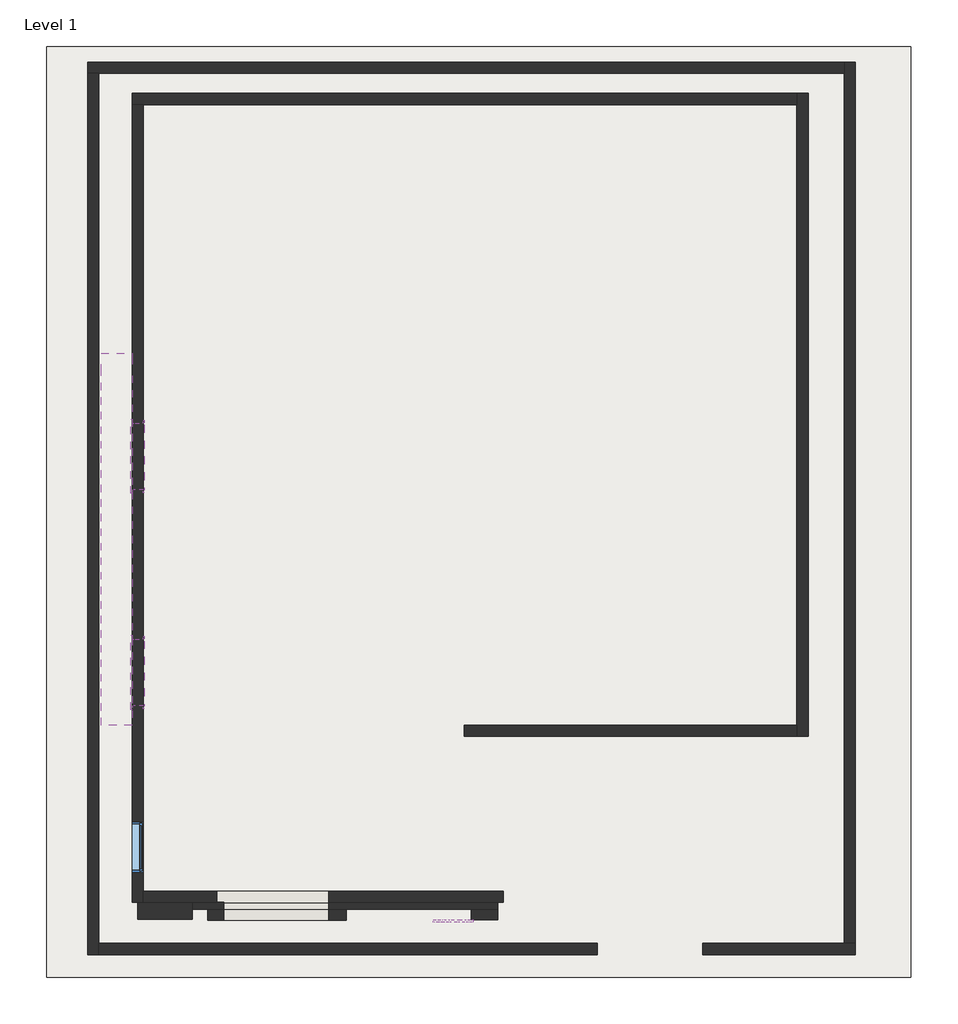
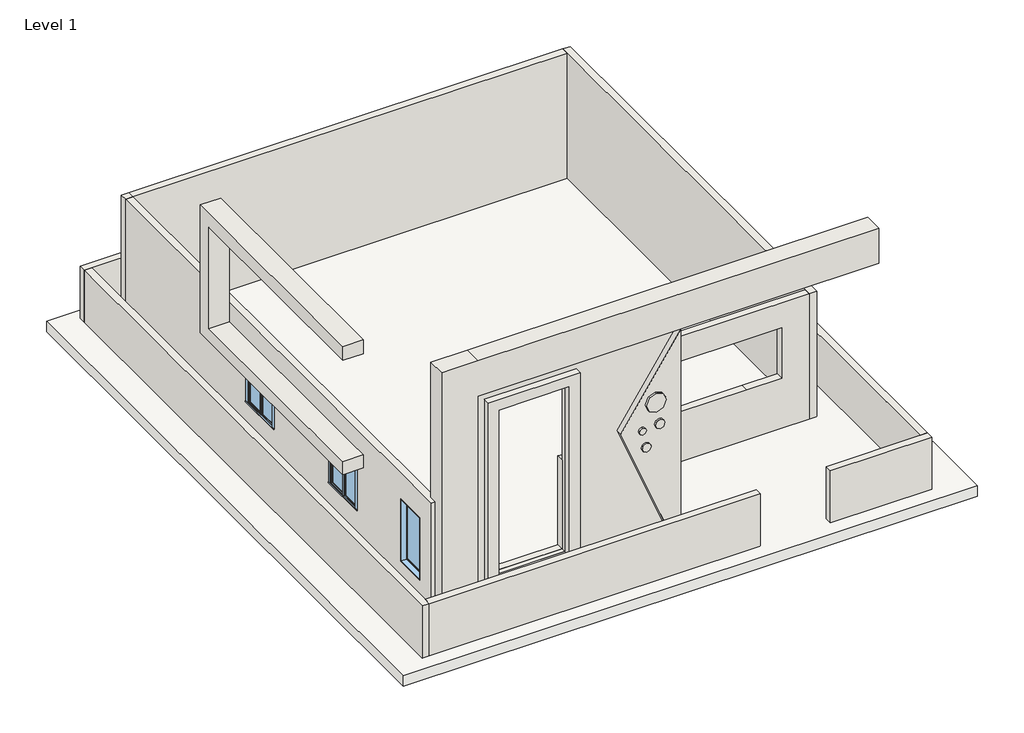
# One storey: 15 walls, 3 windows, 1 slab.
"""IFC4 building model written with IfcOpenShell, lengths in millimetres."""

from ifc_helpers import new_model, si_unit, frame, origin, place, context, project, spatial, polyline, outline, extrude, faceted_brep, transform, mapped, element, save
from components import walls_1_walls_1_592a891f, walls_3_walls_3_f969b8b6, walls_4_walls_4_f4f7f16f, walls_5_walls_5_14261912, walls_6_walls_6_dde418cc, walls_7_walls_7_556ff675, window_0862ab64, window_9a779fa2

model = new_model("IFC4")

# Units and contexts
model_context = context("Model", 3, world=origin())
ifc_project = project(units=[si_unit("LENGTHUNIT", "METRE", prefix="MILLI")], contexts=[model_context])

# Site, building, storey
site = spatial("IfcSite", under=ifc_project)
building = spatial("IfcBuilding", under=site)
storey = spatial("IfcBuildingStorey", under=building, Name="Level 1", Elevation=0.0)

# Slab
placement = place(None, origin())
element("IfcSlab", 1, ObjectType="Generic - 12\"", at=placement, inside=storey, context=model_context, shape_type="SweptSolid", body=[
    extrude(outline(polyline([(5705.2565279, 11449.004673), (5705.2565279, -5619.795327), (-10144.3434721, -5619.795327), (-10144.3434721, 11449.004673), (5705.2565279, 11449.004673)])), frame((0.0, 0.0, -304.8), z_axis=(0.0, 0.0, 1.0), x_axis=(1.0, 0.0, 0.0)), (0.0, 0.0, 1.0), 304.8),
])

# Walls
element("IfcWall", 2, ObjectType="Generic - 8\"", at=placement, inside=storey, context=model_context, shape_type="Brep", body=[
    faceted_brep([(-8577.2311901, 10384.6860488, 0.0), (-8374.0311901, 10384.6860488, 0.0), (3614.7688099, 10384.6860488, 0.0), (3614.7688099, 10384.6860488, 3657.6), (-8374.0311901, 10384.6860488, 3657.6), (-8577.2311901, 10384.6860488, 3657.6), (-8577.2311901, 10587.8860488, 0.0), (-8577.2311901, 10587.8860488, 3657.6), (-8374.0311901, 10587.8860488, 3657.6), (3614.7688099, 10587.8860488, 3657.6), (3614.7688099, 10587.8860488, 0.0)], [[[0, 1, 2, 3, 4, 5]], [[6, 7, 8, 9, 10]], [[2, 1, 0, 6, 10]], [[0, 5, 7, 6]], [[3, 2, 10, 9]], [[5, 4, 8, 7]], [[4, 3, 9, 8]]]),
])
element("IfcWall", 3, ObjectType="Generic - 8\"", at=placement, inside=storey, context=model_context, shape_type="Brep", body=[
    faceted_brep([(-8374.0311901, -4245.7139512, 0.0), (-8374.0311901, -4042.5139512, 0.0), (-8374.0311901, 10384.6860488, 0.0), (-8374.0311901, 10384.6860488, 3657.6), (-8374.0311901, -4042.5139512, 3657.6), (-8374.0311901, -4245.7139512, 3657.6), (-8374.0311901, -3686.9139512, 2900.7966345), (-8374.0311901, -2772.5139512, 2900.7966345), (-8374.0311901, -2772.5139512, 1071.9966345), (-8374.0311901, -3686.9139512, 1071.9966345), (-8374.0311901, 4542.6860488, 2485.5847354), (-8374.0311901, 4542.6860488, 1266.3847354), (-8374.0311901, 3323.4860488, 1266.3847354), (-8374.0311901, 3323.4860488, 2485.5847354), (-8374.0311901, 580.2860488, 2522.8889162), (-8374.0311901, 580.2860488, 1303.6889162), (-8374.0311901, -638.9139512, 1303.6889162), (-8374.0311901, -638.9139512, 2522.8889162), (-8577.2311901, -4245.7139512, 0.0), (-8577.2311901, -4245.7139512, 3657.6), (-8577.2311901, 10384.6860488, 3657.6), (-8577.2311901, 10384.6860488, 0.0), (-8577.2311901, -3686.9139512, 2900.7966345), (-8577.2311901, -3686.9139512, 1071.9966345), (-8577.2311901, -2772.5139512, 1071.9966345), (-8577.2311901, -2772.5139512, 2900.7966345), (-8577.2311901, 4542.6860488, 2485.5847354), (-8577.2311901, 3323.4860488, 2485.5847354), (-8577.2311901, 3323.4860488, 1266.3847354), (-8577.2311901, 4542.6860488, 1266.3847354), (-8577.2311901, 580.2860488, 2522.8889162), (-8577.2311901, -638.9139512, 2522.8889162), (-8577.2311901, -638.9139512, 1303.6889162), (-8577.2311901, 580.2860488, 1303.6889162)], [[[0, 1, 2, 3, 4, 5], [6, 7, 8, 9], [10, 11, 12, 13], [14, 15, 16, 17]], [[18, 19, 20, 21], [22, 23, 24, 25], [26, 27, 28, 29], [30, 31, 32, 33]], [[2, 1, 0, 18, 21]], [[5, 4, 3, 20, 19]], [[0, 5, 19, 18]], [[3, 2, 21, 20]], [[23, 22, 6, 9]], [[24, 23, 9, 8]], [[25, 24, 8, 7]], [[22, 25, 7, 6]], [[11, 10, 26, 29]], [[12, 11, 29, 28]], [[13, 12, 28, 27]], [[10, 13, 27, 26]], [[15, 14, 30, 33]], [[16, 15, 33, 32]], [[17, 16, 32, 31]], [[14, 17, 31, 30]]]),
])
element("IfcWall", 4, ObjectType="Generic - 8\"", at=placement, inside=storey, context=model_context, shape_type="Brep", body=[
    faceted_brep([(-1770.0311901, -4042.5139512, 0.0), (-8374.0311901, -4042.5139512, 0.0), (-8374.0311901, -4042.5139512, 3657.6), (-7057.7216902, -4042.5139512, 3657.6), (-7024.8824762, -4042.5139512, 3657.6), (-7024.8824762, -4042.5139512, 1066.8), (-4972.3150386, -4042.5139512, 1066.8), (-4972.3150386, -4042.5139512, 3657.6), (-4944.6813589, -4042.5139512, 3657.6), (-1871.6311901, -4042.5139512, 3657.6), (-1770.0311901, -4042.5139512, 3657.6), (-1770.0311901, -4245.7139512, 0.0), (-1770.0311901, -4245.7139512, 3657.6), (-1871.6311901, -4245.7139512, 3657.6), (-4944.6813589, -4245.7139512, 3657.6), (-4972.3150386, -4245.7139512, 3657.6), (-4972.3150386, -4245.7139512, 1066.8), (-7024.8824762, -4245.7139512, 1066.8), (-7024.8824762, -4245.7139512, 3657.6), (-7057.7216902, -4245.7139512, 3657.6), (-8374.0311901, -4245.7139512, 3657.6), (-8374.0311901, -4245.7139512, 0.0)], [[[0, 1, 2, 3, 4, 5, 6, 7, 8, 9, 10]], [[11, 12, 13, 14, 15, 16, 17, 18, 19, 20, 21]], [[2, 1, 21, 20]], [[1, 0, 11, 21]], [[0, 10, 12, 11]], [[4, 3, 2, 20, 19, 18]], [[5, 4, 18, 17]], [[6, 5, 17, 16]], [[7, 6, 16, 15]], [[9, 8, 7, 15, 14, 13]], [[10, 9, 13, 12]]]),
])
element("IfcWall", 5, ObjectType="Generic - 8\"", at=placement, inside=storey, context=model_context, shape_type="Brep", body=[
    faceted_brep([(3614.7688099, 10587.8860488, 0.0), (3614.7688099, 10384.6860488, 0.0), (3614.7688099, -994.5139512, 0.0), (3614.7688099, -1197.7139512, 0.0), (3614.7688099, -1197.7139512, 3657.6), (3614.7688099, -994.5139512, 3657.6), (3614.7688099, 10384.6860488, 3657.6), (3614.7688099, 10587.8860488, 3657.6), (3817.9688099, 10587.8860488, 0.0), (3817.9688099, 10587.8860488, 3657.6), (3817.9688099, -1197.7139512, 3657.6), (3817.9688099, -1197.7139512, 0.0)], [[[0, 1, 2, 3, 4, 5, 6, 7]], [[8, 9, 10, 11]], [[3, 2, 1, 0, 8, 11]], [[0, 7, 9, 8]], [[7, 6, 5, 4, 10, 9]], [[4, 3, 11, 10]]]),
])
element("IfcWall", 6, ObjectType="Generic - 8\"", at=placement, inside=storey, context=model_context, shape_type="SweptSolid", body=[
    extrude(outline(polyline([(0.0, 3614.7688099), (3657.6, 3614.7688099), (3657.6, -2481.2311901), (0.0, -2481.2311901), (0.0, 3614.7688099)]), holes=[polyline([(2930.097392, 2852.2278443), (1465.048696, 2852.2278443), (1465.048696, 1887.5688099), (1465.048696, -1052.1762723), (2930.097392, -1052.1762723), (2930.097392, 2852.2278443)])]), frame((0.0, -1197.7139512, 0.0), z_axis=(0.0, 1.0, 0.0), x_axis=(0.0, 0.0, 1.0)), (0.0, 0.0, 1.0), 203.2),
])
element("IfcWall", 7, ObjectType="Generic - 8\"", at=placement, inside=storey, context=model_context, shape_type="Brep", body=[
    faceted_brep([(-9386.1684306, 10954.9442531, 0.0), (-9182.9684306, 10954.9442531, 0.0), (4482.2315694, 10954.9442531, 0.0), (4482.2315694, 10954.9442531, 1524.0), (-9182.9684306, 10954.9442531, 1524.0), (-9386.1684306, 10954.9442531, 1524.0), (-9386.1684306, 11158.1442531, 0.0), (-9386.1684306, 11158.1442531, 1524.0), (4482.2315694, 11158.1442531, 1524.0), (4482.2315694, 11158.1442531, 0.0)], [[[0, 1, 2, 3, 4, 5]], [[6, 7, 8, 9]], [[2, 1, 0, 6, 9]], [[5, 4, 3, 8, 7]], [[0, 5, 7, 6]], [[3, 2, 9, 8]]]),
])
element("IfcWall", 8, ObjectType="Generic - 8\"", at=placement, inside=storey, context=model_context, shape_type="Brep", body=[
    faceted_brep([(-9182.9684306, -5199.4557469, 0.0), (-9182.9684306, -4996.2557469, 0.0), (-9182.9684306, 10954.9442531, 0.0), (-9182.9684306, 10954.9442531, 1524.0), (-9182.9684306, -4996.2557469, 1524.0), (-9182.9684306, -5199.4557469, 1524.0), (-9386.1684306, -5199.4557469, 0.0), (-9386.1684306, -5199.4557469, 1524.0), (-9386.1684306, 10954.9442531, 1524.0), (-9386.1684306, 10954.9442531, 0.0)], [[[0, 1, 2, 3, 4, 5]], [[6, 7, 8, 9]], [[2, 1, 0, 6, 9]], [[5, 4, 3, 8, 7]], [[0, 5, 7, 6]], [[3, 2, 9, 8]]]),
])
element("IfcWall", 9, ObjectType="Generic - 8\"", at=placement, inside=storey, context=model_context, shape_type="Brep", body=[
    faceted_brep([(-9182.9684306, -4996.2557469, 1524.0), (-42.8311901, -4996.2557469, 1524.0), (-42.8311901, -4996.2557469, 0.0), (-9182.9684306, -4996.2557469, 0.0), (-9182.9684306, -5199.4557469, 1524.0), (-9182.9684306, -5199.4557469, 0.0), (-42.8311901, -5199.4557469, 0.0), (-42.8311901, -5199.4557469, 1524.0)], [[[0, 1, 2, 3]], [[4, 5, 6, 7]], [[0, 3, 5, 4]], [[1, 0, 4, 7]], [[2, 1, 7, 6]], [[3, 2, 6, 5]]]),
    faceted_brep([(4685.4315694, -4996.2557469, 0.0), (4482.2315694, -4996.2557469, 0.0), (1887.5688099, -4996.2557469, 0.0), (1887.5688099, -4996.2557469, 1524.0), (4482.2315694, -4996.2557469, 1524.0), (4685.4315694, -4996.2557469, 1524.0), (4685.4315694, -5199.4557469, 0.0), (4685.4315694, -5199.4557469, 1524.0), (1887.5688099, -5199.4557469, 1524.0), (1887.5688099, -5199.4557469, 0.0)], [[[0, 1, 2, 3, 4, 5]], [[6, 7, 8, 9]], [[0, 5, 7, 6]], [[2, 1, 0, 6, 9]], [[3, 2, 9, 8]], [[5, 4, 3, 8, 7]]]),
])
element("IfcWall", 10, ObjectType="Generic - 8\"", at=placement, inside=storey, context=model_context, shape_type="Brep", body=[
    faceted_brep([(4482.2315694, 11158.1442531, 0.0), (4482.2315694, 10954.9442531, 0.0), (4482.2315694, -4996.2557469, 0.0), (4482.2315694, -4996.2557469, 1524.0), (4482.2315694, 10954.9442531, 1524.0), (4482.2315694, 11158.1442531, 1524.0), (4685.4315694, 11158.1442531, 0.0), (4685.4315694, 11158.1442531, 1524.0), (4685.4315694, -4996.2557469, 1524.0), (4685.4315694, -4996.2557469, 0.0)], [[[0, 1, 2, 3, 4, 5]], [[6, 7, 8, 9]], [[2, 1, 0, 6, 9]], [[5, 4, 3, 8, 7]], [[0, 5, 7, 6]], [[3, 2, 9, 8]]]),
])
walls_1_walls_1_shape = walls_1_walls_1_592a891f(model_context)
element("IfcWall", 11, ObjectType="Walls 1 : Walls 1", at=placement, inside=storey, context=model_context, shape_type="MappedRepresentation", body=[
    mapped(walls_1_walls_1_shape, transform((0.0, 0.0, 0.0), x_axis=(1.0, 0.0, 0.0), y_axis=(0.0, 1.0, 0.0), z_axis=(0.0, 0.0, 1.0))),
])
walls_3_walls_3_shape = walls_3_walls_3_f969b8b6(model_context)
element("IfcWall", 12, ObjectType="Walls 3 : Walls 3", at=placement, inside=storey, context=model_context, shape_type="MappedRepresentation", body=[
    mapped(walls_3_walls_3_shape, transform((0.0, 0.0, 0.0), x_axis=(1.0, 0.0, 0.0), y_axis=(0.0, 1.0, 0.0), z_axis=(0.0, 0.0, 1.0))),
])
walls_4_walls_4_shape = walls_4_walls_4_f4f7f16f(model_context)
element("IfcWall", 13, ObjectType="Walls 4 : Walls 4", at=placement, inside=storey, context=model_context, shape_type="MappedRepresentation", body=[
    mapped(walls_4_walls_4_shape, transform((0.0, 0.0, 0.0), x_axis=(1.0, 0.0, 0.0), y_axis=(0.0, 1.0, 0.0), z_axis=(0.0, 0.0, 1.0))),
])
walls_5_walls_5_shape = walls_5_walls_5_14261912(model_context)
element("IfcWall", 14, ObjectType="Walls 5 : Walls 5", at=placement, inside=storey, context=model_context, shape_type="MappedRepresentation", body=[
    mapped(walls_5_walls_5_shape, transform((0.0, 0.0, 0.0), x_axis=(1.0, 0.0, 0.0), y_axis=(0.0, 1.0, 0.0), z_axis=(0.0, 0.0, 1.0))),
])
walls_6_walls_6_shape = walls_6_walls_6_dde418cc(model_context)
element("IfcWall", 15, ObjectType="Walls 6 : Walls 6", at=placement, inside=storey, context=model_context, shape_type="MappedRepresentation", body=[
    mapped(walls_6_walls_6_shape, transform((0.0, 0.0, 0.0), x_axis=(1.0, 0.0, 0.0), y_axis=(0.0, 1.0, 0.0), z_axis=(0.0, 0.0, 1.0))),
])
walls_7_walls_7_shape = walls_7_walls_7_556ff675(model_context)
element("IfcWall", 16, ObjectType="Walls 7 : Walls 7", at=placement, inside=storey, context=model_context, shape_type="MappedRepresentation", body=[
    mapped(walls_7_walls_7_shape, transform((0.0, 0.0, 0.0), x_axis=(1.0, 0.0, 0.0), y_axis=(0.0, 1.0, 0.0), z_axis=(0.0, 0.0, 1.0))),
])

# Windows
window_shape = window_0862ab64(model_context)
element("IfcWindow", 17, ObjectType="Casement Dbl with Trim : 48\" x 48\"", at=placement, inside=storey, context=model_context, shape_type="MappedRepresentation", body=[
    mapped(window_shape, transform((-8456.5811901, 3933.0860488, 351.9847354), x_axis=(0.0, 1.0, 0.0), y_axis=(-1.0, 0.0, 0.0), z_axis=(0.0, 0.0, 1.0))),
])
element("IfcWindow", 18, ObjectType="Casement Dbl with Trim : 48\" x 48\"", at=placement, inside=storey, context=model_context, shape_type="MappedRepresentation", body=[
    mapped(window_shape, transform((-8456.5811901, -29.3139512, 389.2889162), x_axis=(0.0, 1.0, 0.0), y_axis=(-1.0, 0.0, 0.0), z_axis=(0.0, 0.0, 1.0))),
])
window_2_shape = window_9a779fa2(model_context)
element("IfcWindow", 19, ObjectType="Fixed : 36\" x 72\"", at=placement, inside=storey, context=model_context, shape_type="MappedRepresentation", body=[
    mapped(window_2_shape, transform((-8475.6311901, -3267.8139512, 767.1966345), x_axis=(0.0, -1.0, 0.0), y_axis=(1.0, 0.0, 0.0), z_axis=(0.0, 0.0, 1.0))),
])

save(model, "model.ifc")

# Revit data of these elements
# Type "Generic - 12\""
#   Assembly Code = "B1010"
#   Function = 0
#   Layers, outside or top first: 1' - 0" no material (function 1)
# Type "Generic - 8\""
#   Assembly Code = "B2010"
#   Layers, outside or top first: 0' - 8" no material (function 1)
# Type "Casement Dbl with Trim : 48\" x 48\""
#   Type Mark = "10"
#   Construction Type Id = "GSP4R"
#   Assembly Code = "B2020100"
#   Analytic Construction = "1/8 in Pilkington single glazing"
#   Visual Light Transmittance = 0.9
#   Thermal Resistance (R) = 1.53941 (h·ft²·°F)/BTU
#   Solar Heat Gain Coefficient = 0.78
#   Heat Transfer Coefficient (U) = 0.6496 BTU/(h·ft²·°F)
#   Height = 4' - 0"
#   Default Sill Height = 3' - 0"
#   Trim Projection - Ext. = 0' - 0 1/2"
#   Trim Projection - Int. = 0' - 0 3/4"
#   Trim Width - Exterior = 0' - 3 1/2"
#   Trim Width - Interior = 0' - 3 1/2"
#   Width = 4' - 0"
#   Window Inset = 0' - 0 3/4"
#   Define Thermal Properties by = 1
#   Glass Pane Material = Glass
#   Sash Material = Sash
#   Trim Exterior Material = Trim
#   Trim Interior Material = Trim
#   Wall Closure = (empty or 0)
# Type "Fixed : 36\" x 72\""
#   Type Mark = "9"
#   Construction Type Id = "GSP4R"
#   Assembly Code = "B2020100"
#   Analytic Construction = "1/8 in Pilkington single glazing"
#   Visual Light Transmittance = 0.9
#   Solar Heat Gain Coefficient = 0.78
#   Heat Transfer Coefficient (U) = 0.6496 BTU/(h·ft²·°F)
#   Height = 6' - 0"
#   Default Sill Height = 1' - 0"
#   Width = 3' - 0"
#   Window Inset = 0' - 0 3/4"
#   Define Thermal Properties by = 1
#   Glass Pane Material = Glass
#   Sash Material = Sash
#   Wall Closure = (empty or 0)
# Element 1 (IfcSlab, "Generic - 12\"")
#   Height Offset From Level = 0' - 0"
#   Phase Created = New Construction
#   Materials on its faces: "Default Floor"
# Elements 2, 3, 4, 5, 6 (IfcWall, "Generic - 8\"")
#   Top Offset = 0' - 0"
#   Base Offset = 0' - 0"
#   Unconnected Height = 12' - 0"
#   wall height = 12' - 0"
#   Phase Created = New Construction
#   Base Constraint = Level 1
#   Materials on its faces: "Default Wall"
# Elements 7, 8, 9, 10 (IfcWall, "Generic - 8\"")
#   Top Offset = 0' - 0"
#   Base Offset = 0' - 0"
#   Unconnected Height = 5' - 0"
#   wall height = 5' - 0"
#   Phase Created = New Construction
#   Base Constraint = Level 1
#   Materials on its faces: "Default Wall"
# Element 11 (IfcWall, "Walls 1 : Walls 1")
#   Phase Created = New Construction
#   Materials on its faces: "Default Wall"
# Element 12 (IfcWall, "Walls 3 : Walls 3")
#   Phase Created = New Construction
#   Materials on its faces: "Default Wall"
# Element 13 (IfcWall, "Walls 4 : Walls 4")
#   Phase Created = New Construction
#   Materials on its faces: "Default Wall"
# Element 14 (IfcWall, "Walls 5 : Walls 5")
#   Phase Created = New Construction
#   Materials on its faces: "Default Wall"
# Element 15 (IfcWall, "Walls 6 : Walls 6")
#   Phase Created = New Construction
#   Materials on its faces: "Default Wall"
# Element 16 (IfcWall, "Walls 7 : Walls 7")
#   Phase Created = New Construction
#   Materials on its faces: "Default Wall"
# Element 17 (IfcWindow, "Casement Dbl with Trim : 48\" x 48\"")
#   Mark = "6"
#   Phase Created = New Construction
#   Materials on its faces: "Sash", "Trim", "Glass"
# Element 18 (IfcWindow, "Casement Dbl with Trim : 48\" x 48\"")
#   Mark = "7"
#   Phase Created = New Construction
#   Materials on its faces: "Sash", "Trim", "Glass"
# Element 19 (IfcWindow, "Fixed : 36\" x 72\"")
#   Mark = "2"
#   Phase Created = New Construction
#   Materials on its faces: "Sash", "Glass"
# Materials
#   "Glass": class "Glass", colour RGB 0 128 192, transparency 0.75, Description = "Soda Lime Glass", Cost = 0
#   "Sash": class "Wood", colour RGB 224 178 126, transparency 0
#   "Trim": class "Wood", colour RGB 224 178 126, transparency 0
#   "Default Floor": colour RGB 128 128 128, transparency 0
#   "Default Wall": colour RGB 128 128 128, transparency 0
